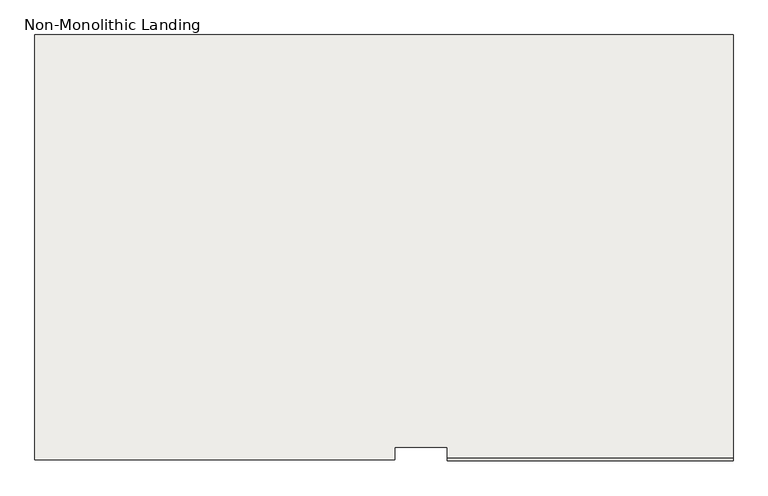
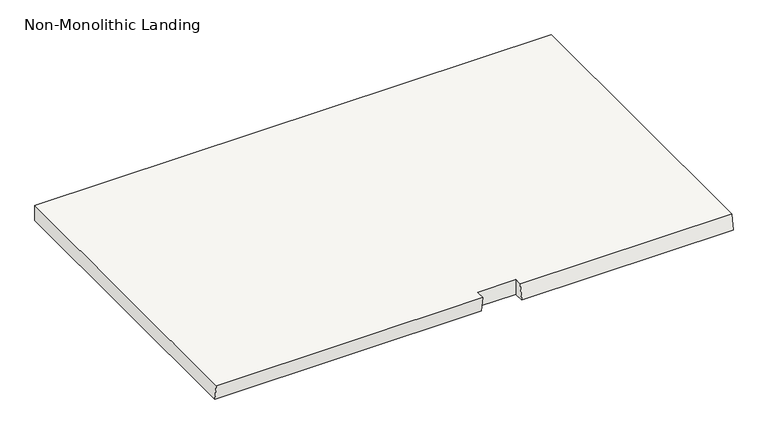
"""IFC4 building model written with IfcOpenShell, lengths in millimetres: slab geometry, Non-Monolithic Landing."""

from ifc_helpers import new_model, si_unit, origin, place, context, project, spatial, faceted_brep, source, transform, mapped, element, save


def non_monolithic_landing_8206a9fb(model_context):
    return source(origin(), model_context, "Body", "Brep", [
        faceted_brep([(602.1868738, 7326.2805518, 1739.1304348), (602.1868738, 7319.0930518, 1689.1304348), (1275.5786001, 7319.0930518, 1689.1304348), (1275.5786001, 7326.2805518, 1739.1304348), (479.5868738, 7321.4805518, 1739.1304348), (479.5868738, 7351.2805518, 1739.1304348), (602.1868738, 7351.2805518, 1739.1304348), (1275.5786001, 7351.2805518, 1739.1304348), (1275.5786001, 8321.5063331, 1739.1304348), (-368.0389075, 8321.5063331, 1739.1304348), (-368.0389075, 7321.4805518, 1739.1304348), (602.1868738, 7351.2805518, 1689.1304348), (479.5868738, 7351.2805518, 1689.1304348), (479.5868738, 7328.6680518, 1689.1304348), (-368.0389075, 7328.6680518, 1689.1304348), (-368.0389075, 8321.5063331, 1689.1304348), (1275.5786001, 8321.5063331, 1689.1304348), (1275.5786001, 7351.2805518, 1689.1304348)], [[[0, 1, 2, 3]], [[4, 5, 6, 0, 3, 7, 8, 9, 10]], [[11, 12, 13, 14, 15, 16, 17, 2, 1]], [[5, 4, 13, 12]], [[6, 5, 12, 11]], [[0, 6, 11, 1]], [[7, 3, 2, 17]], [[8, 7, 17, 16]], [[9, 8, 16, 15]], [[10, 9, 15, 14]], [[4, 10, 14, 13]]]),
    ])


if __name__ == "__main__":
    model = new_model("IFC4")
    model_context = context("Model", 3, world=origin())
    ifc_project = project(units=[si_unit("LENGTHUNIT", "METRE", prefix="MILLI")], contexts=[model_context])
    site = spatial("IfcSite", under=ifc_project)
    building = spatial("IfcBuilding", under=site)
    placement = place(None, origin())
    non_monolithic_landing_shape = non_monolithic_landing_8206a9fb(model_context)
    element("IfcSlab", 1, ObjectType="Non-Monolithic Landing", at=placement, inside=building, context=model_context, shape_type="MappedRepresentation", body=[
        mapped(non_monolithic_landing_shape, transform((0.0, 0.0, 0.0), x_axis=(1.0, 0.0, 0.0), y_axis=(0.0, 1.0, 0.0), z_axis=(0.0, 0.0, 1.0))),
    ])
    save(model, "model.ifc")
